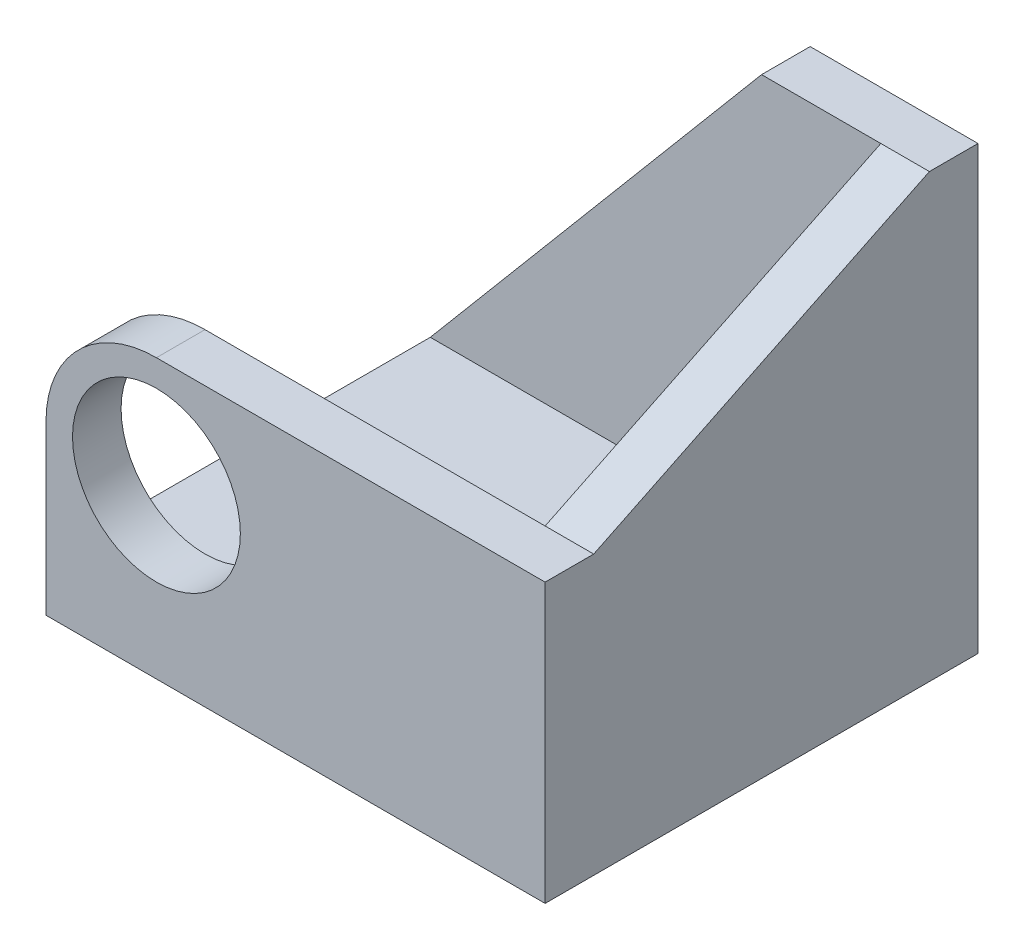
ISO-10303-21;
HEADER;
FILE_DESCRIPTION(('STEP AP214'),'2;1');
FILE_NAME('part.step','',(''),(''),'','','');
FILE_SCHEMA(('AUTOMOTIVE_DESIGN { 1 0 10303 214 1 1 1 1 }'));
ENDSEC;
DATA;
#1=APPLICATION_CONTEXT('core data for automotive mechanical design processes');
#2=APPLICATION_PROTOCOL_DEFINITION('international standard','automotive_design',2000,#1);
#3=PRODUCT_CONTEXT('',#1,'mechanical');
#4=PRODUCT('Part','Part','',(#3));
#5=PRODUCT_RELATED_PRODUCT_CATEGORY('part','',(#4));
#6=PRODUCT_DEFINITION_FORMATION('','',#4);
#7=PRODUCT_DEFINITION_CONTEXT('part definition',#1,'design');
#8=PRODUCT_DEFINITION('design','',#6,#7);
#9=PRODUCT_DEFINITION_SHAPE('','',#8);
#10=(LENGTH_UNIT() NAMED_UNIT(*) SI_UNIT(.MILLI.,.METRE.));
#11=(NAMED_UNIT(*) PLANE_ANGLE_UNIT() SI_UNIT($,.RADIAN.));
#12=(NAMED_UNIT(*) SI_UNIT($,.STERADIAN.) SOLID_ANGLE_UNIT());
#13=UNCERTAINTY_MEASURE_WITH_UNIT(LENGTH_MEASURE(1.E-05),#10,'distance_accuracy_value','');
#14=(GEOMETRIC_REPRESENTATION_CONTEXT(3) GLOBAL_UNCERTAINTY_ASSIGNED_CONTEXT((#13)) GLOBAL_UNIT_ASSIGNED_CONTEXT((#10,
#11,#12)) REPRESENTATION_CONTEXT('',''));
#15=CARTESIAN_POINT('',(0.,0.,0.));
#16=DIRECTION('',(0.,0.,1.));
#17=DIRECTION('',(1.,0.,0.));
#18=AXIS2_PLACEMENT_3D('',#15,#16,#17);
#19=CARTESIAN_POINT('',(25.,38.,0.));
#20=DIRECTION('',(0.,0.,1.));
#21=DIRECTION('',(1.,0.,0.));
#22=AXIS2_PLACEMENT_3D('',#19,#20,#21);
#23=PLANE('',#22);
#24=CARTESIAN_POINT('',(25.,38.,0.));
#25=DIRECTION('',(0.,0.,1.));
#26=DIRECTION('',(1.,0.,0.));
#27=AXIS2_PLACEMENT_3D('',#24,#25,#26);
#28=CIRCLE('',#27,19.);
#29=CARTESIAN_POINT('',(44.,38.,0.));
#30=VERTEX_POINT('',#29);
#31=EDGE_CURVE('E269',#30,#30,#28,.T.);
#32=ORIENTED_EDGE('',*,*,#31,.T.);
#33=EDGE_LOOP('',(#32));
#34=FACE_BOUND('',#33,.T.);
#35=DIRECTION('',(0.,-1.,0.));
#36=VECTOR('',#35,1.);
#37=CARTESIAN_POINT('',(67.,27.,0.));
#38=LINE('',#37,#36);
#39=CARTESIAN_POINT('',(67.,27.,0.));
#40=VERTEX_POINT('',#39);
#41=CARTESIAN_POINT('',(67.,11.,0.));
#42=VERTEX_POINT('',#41);
#43=EDGE_CURVE('E257',#40,#42,#38,.T.);
#44=ORIENTED_EDGE('',*,*,#43,.T.);
#45=DIRECTION('',(-1.,0.,0.));
#46=VECTOR('',#45,1.);
#47=CARTESIAN_POINT('',(0.,11.,0.));
#48=LINE('',#47,#46);
#49=CARTESIAN_POINT('',(0.,11.,0.));
#50=VERTEX_POINT('',#49);
#51=EDGE_CURVE('E164',#42,#50,#48,.T.);
#52=ORIENTED_EDGE('',*,*,#51,.T.);
#53=DIRECTION('',(0.,-1.,0.));
#54=VECTOR('',#53,1.);
#55=CARTESIAN_POINT('',(0.,0.,0.));
#56=LINE('',#55,#54);
#57=CARTESIAN_POINT('',(0.,38.,0.));
#58=VERTEX_POINT('',#57);
#59=EDGE_CURVE('E123',#58,#50,#56,.T.);
#60=ORIENTED_EDGE('',*,*,#59,.F.);
#61=CARTESIAN_POINT('',(25.,38.,0.));
#62=DIRECTION('',(0.,0.,1.));
#63=DIRECTION('',(1.,0.,0.));
#64=AXIS2_PLACEMENT_3D('',#61,#62,#63);
#65=CIRCLE('',#64,25.);
#66=CARTESIAN_POINT('',(25.,63.,0.));
#67=VERTEX_POINT('',#66);
#68=EDGE_CURVE('E81',#67,#58,#65,.T.);
#69=ORIENTED_EDGE('',*,*,#68,.F.);
#70=DIRECTION('',(-1.,0.,0.));
#71=VECTOR('',#70,1.);
#72=CARTESIAN_POINT('',(113.,63.,0.));
#73=LINE('',#72,#71);
#74=CARTESIAN_POINT('',(102.,63.,0.));
#75=VERTEX_POINT('',#74);
#76=EDGE_CURVE('E129',#75,#67,#73,.T.);
#77=ORIENTED_EDGE('',*,*,#76,.F.);
#78=DIRECTION('',(0.,-1.,0.));
#79=VECTOR('',#78,1.);
#80=CARTESIAN_POINT('',(102.,63.,0.));
#81=LINE('',#80,#79);
#82=CARTESIAN_POINT('',(102.,27.,0.));
#83=VERTEX_POINT('',#82);
#84=EDGE_CURVE('E185',#75,#83,#81,.T.);
#85=ORIENTED_EDGE('',*,*,#84,.T.);
#86=DIRECTION('',(1.,0.,0.));
#87=VECTOR('',#86,1.);
#88=CARTESIAN_POINT('',(102.,27.,0.));
#89=LINE('',#88,#87);
#90=EDGE_CURVE('E249',#40,#83,#89,.T.);
#91=ORIENTED_EDGE('',*,*,#90,.F.);
#92=EDGE_LOOP('',(#44,#52,#60,#69,#77,#85,#91));
#93=FACE_BOUND('',#92,.T.);
#94=ADVANCED_FACE('F44',(#34,#93),#23,.F.);
#95=CARTESIAN_POINT('',(102.,0.,0.));
#96=DIRECTION('',(1.,0.,0.));
#97=DIRECTION('',(0.,0.,-1.));
#98=AXIS2_PLACEMENT_3D('',#95,#96,#97);
#99=PLANE('',#98);
#100=DIRECTION('',(0.,0.,-1.));
#101=VECTOR('',#100,1.);
#102=CARTESIAN_POINT('',(102.,27.,-76.));
#103=LINE('',#102,#101);
#104=CARTESIAN_POINT('',(102.,27.,-76.));
#105=VERTEX_POINT('',#104);
#106=EDGE_CURVE('E256',#83,#105,#103,.T.);
#107=ORIENTED_EDGE('',*,*,#106,.F.);
#108=ORIENTED_EDGE('',*,*,#84,.F.);
#109=DIRECTION('',(0.,-0.437724250235496,0.899109270753991));
#110=VECTOR('',#109,1.);
#111=CARTESIAN_POINT('',(102.,100.,-76.));
#112=LINE('',#111,#110);
#113=CARTESIAN_POINT('',(102.,100.,-76.));
#114=VERTEX_POINT('',#113);
#115=EDGE_CURVE('E189',#114,#75,#112,.T.);
#116=ORIENTED_EDGE('',*,*,#115,.F.);
#117=DIRECTION('',(0.,1.,0.));
#118=VECTOR('',#117,1.);
#119=CARTESIAN_POINT('',(102.,0.,-76.));
#120=LINE('',#119,#118);
#121=EDGE_CURVE('E184',#105,#114,#120,.T.);
#122=ORIENTED_EDGE('',*,*,#121,.F.);
#123=EDGE_LOOP('',(#107,#108,#116,#122));
#124=FACE_BOUND('',#123,.T.);
#125=ADVANCED_FACE('F284',(#124),#99,.F.);
#126=CARTESIAN_POINT('',(0.,0.,-76.));
#127=DIRECTION('',(0.,0.,1.));
#128=DIRECTION('',(1.,0.,0.));
#129=AXIS2_PLACEMENT_3D('',#126,#127,#128);
#130=PLANE('',#129);
#131=DIRECTION('',(1.,0.,0.));
#132=VECTOR('',#131,1.);
#133=CARTESIAN_POINT('',(102.,11.,-76.));
#134=LINE('',#133,#132);
#135=CARTESIAN_POINT('',(0.,11.,-76.));
#136=VERTEX_POINT('',#135);
#137=CARTESIAN_POINT('',(67.,11.,-76.));
#138=VERTEX_POINT('',#137);
#139=EDGE_CURVE('E270',#136,#138,#134,.T.);
#140=ORIENTED_EDGE('',*,*,#139,.T.);
#141=DIRECTION('',(0.,-1.,0.));
#142=VECTOR('',#141,1.);
#143=CARTESIAN_POINT('',(67.,27.,-76.));
#144=LINE('',#143,#142);
#145=CARTESIAN_POINT('',(67.,27.,-76.));
#146=VERTEX_POINT('',#145);
#147=EDGE_CURVE('E58',#146,#138,#144,.T.);
#148=ORIENTED_EDGE('',*,*,#147,.F.);
#149=DIRECTION('',(-1.,0.,0.));
#150=VECTOR('',#149,1.);
#151=CARTESIAN_POINT('',(67.,27.,-76.));
#152=LINE('',#151,#150);
#153=EDGE_CURVE('E254',#105,#146,#152,.T.);
#154=ORIENTED_EDGE('',*,*,#153,.F.);
#155=ORIENTED_EDGE('',*,*,#121,.T.);
#156=DIRECTION('',(1.,0.,0.));
#157=VECTOR('',#156,1.);
#158=CARTESIAN_POINT('',(113.,100.,-76.));
#159=LINE('',#158,#157);
#160=CARTESIAN_POINT('',(75.,100.,-76.));
#161=VERTEX_POINT('',#160);
#162=EDGE_CURVE('E158',#161,#114,#159,.T.);
#163=ORIENTED_EDGE('',*,*,#162,.F.);
#164=DIRECTION('',(0.64440029083596,0.764688345125339,0.));
#165=VECTOR('',#164,1.);
#166=CARTESIAN_POINT('',(75.,100.,-76.));
#167=LINE('',#166,#165);
#168=EDGE_CURVE('E162',#136,#161,#167,.T.);
#169=ORIENTED_EDGE('',*,*,#168,.F.);
#170=EDGE_LOOP('',(#140,#148,#154,#155,#163,#169));
#171=FACE_BOUND('',#170,.T.);
#172=ADVANCED_FACE('F275',(#171),#130,.T.);
#173=CARTESIAN_POINT('',(0.,11.,0.));
#174=DIRECTION('',(0.,1.,0.));
#175=DIRECTION('',(0.,0.,1.));
#176=AXIS2_PLACEMENT_3D('',#173,#174,#175);
#177=PLANE('',#176);
#178=ORIENTED_EDGE('',*,*,#51,.F.);
#179=DIRECTION('',(0.,0.,1.));
#180=VECTOR('',#179,1.);
#181=CARTESIAN_POINT('',(67.,11.,0.));
#182=LINE('',#181,#180);
#183=EDGE_CURVE('E251',#138,#42,#182,.T.);
#184=ORIENTED_EDGE('',*,*,#183,.F.);
#185=ORIENTED_EDGE('',*,*,#139,.F.);
#186=DIRECTION('',(0.,0.,-1.));
#187=VECTOR('',#186,1.);
#188=CARTESIAN_POINT('',(0.,11.,-76.));
#189=LINE('',#188,#187);
#190=EDGE_CURVE('E227',#50,#136,#189,.T.);
#191=ORIENTED_EDGE('',*,*,#190,.F.);
#192=EDGE_LOOP('',(#178,#184,#185,#191));
#193=FACE_BOUND('',#192,.T.);
#194=ADVANCED_FACE('F273',(#193),#177,.T.);
#195=CARTESIAN_POINT('',(0.,0.,11.));
#196=DIRECTION('',(1.,0.,0.));
#197=DIRECTION('',(0.,1.,0.));
#198=AXIS2_PLACEMENT_3D('',#195,#196,#197);
#199=PLANE('',#198);
#200=ORIENTED_EDGE('',*,*,#59,.T.);
#201=ORIENTED_EDGE('',*,*,#190,.T.);
#202=DIRECTION('',(0.,0.,1.));
#203=VECTOR('',#202,1.);
#204=CARTESIAN_POINT('',(0.,11.,-87.));
#205=LINE('',#204,#203);
#206=CARTESIAN_POINT('',(0.,11.,-87.));
#207=VERTEX_POINT('',#206);
#208=EDGE_CURVE('E177',#207,#136,#205,.T.);
#209=ORIENTED_EDGE('',*,*,#208,.F.);
#210=DIRECTION('',(0.,1.,0.));
#211=VECTOR('',#210,1.);
#212=CARTESIAN_POINT('',(0.,0.,-87.));
#213=LINE('',#212,#211);
#214=CARTESIAN_POINT('',(0.,0.,-87.));
#215=VERTEX_POINT('',#214);
#216=EDGE_CURVE('E152',#215,#207,#213,.T.);
#217=ORIENTED_EDGE('',*,*,#216,.F.);
#218=DIRECTION('',(0.,0.,-1.));
#219=VECTOR('',#218,1.);
#220=CARTESIAN_POINT('',(0.,0.,11.));
#221=LINE('',#220,#219);
#222=CARTESIAN_POINT('',(0.,0.,11.));
#223=VERTEX_POINT('',#222);
#224=EDGE_CURVE('E11',#223,#215,#221,.T.);
#225=ORIENTED_EDGE('',*,*,#224,.F.);
#226=DIRECTION('',(0.,-1.,0.));
#227=VECTOR('',#226,1.);
#228=CARTESIAN_POINT('',(0.,0.,11.));
#229=LINE('',#228,#227);
#230=CARTESIAN_POINT('',(0.,38.,11.));
#231=VERTEX_POINT('',#230);
#232=EDGE_CURVE('E134',#231,#223,#229,.T.);
#233=ORIENTED_EDGE('',*,*,#232,.F.);
#234=DIRECTION('',(0.,0.,-1.));
#235=VECTOR('',#234,1.);
#236=CARTESIAN_POINT('',(0.,38.,11.));
#237=LINE('',#236,#235);
#238=EDGE_CURVE('E122',#231,#58,#237,.T.);
#239=ORIENTED_EDGE('',*,*,#238,.T.);
#240=EDGE_LOOP('',(#200,#201,#209,#217,#225,#233,#239));
#241=FACE_BOUND('',#240,.T.);
#242=ADVANCED_FACE('F50',(#241),#199,.F.);
#243=CARTESIAN_POINT('',(0.,0.,11.));
#244=DIRECTION('',(0.,1.,0.));
#245=DIRECTION('',(0.,0.,1.));
#246=AXIS2_PLACEMENT_3D('',#243,#244,#245);
#247=PLANE('',#246);
#248=ORIENTED_EDGE('',*,*,#224,.T.);
#249=DIRECTION('',(-1.,0.,0.));
#250=VECTOR('',#249,1.);
#251=CARTESIAN_POINT('',(113.,0.,-87.));
#252=LINE('',#251,#250);
#253=CARTESIAN_POINT('',(113.,0.,-87.));
#254=VERTEX_POINT('',#253);
#255=EDGE_CURVE('E143',#254,#215,#252,.T.);
#256=ORIENTED_EDGE('',*,*,#255,.F.);
#257=DIRECTION('',(0.,0.,-1.));
#258=VECTOR('',#257,1.);
#259=CARTESIAN_POINT('',(113.,0.,11.));
#260=LINE('',#259,#258);
#261=CARTESIAN_POINT('',(113.,0.,11.));
#262=VERTEX_POINT('',#261);
#263=EDGE_CURVE('E52',#262,#254,#260,.T.);
#264=ORIENTED_EDGE('',*,*,#263,.F.);
#265=DIRECTION('',(1.,0.,0.));
#266=VECTOR('',#265,1.);
#267=CARTESIAN_POINT('',(0.,0.,11.));
#268=LINE('',#267,#266);
#269=EDGE_CURVE('E91',#223,#262,#268,.T.);
#270=ORIENTED_EDGE('',*,*,#269,.F.);
#271=EDGE_LOOP('',(#248,#256,#264,#270));
#272=FACE_BOUND('',#271,.T.);
#273=ADVANCED_FACE('F147',(#272),#247,.F.);
#274=CARTESIAN_POINT('',(113.,0.,11.));
#275=DIRECTION('',(-1.,0.,0.));
#276=DIRECTION('',(0.,0.,1.));
#277=AXIS2_PLACEMENT_3D('',#274,#275,#276);
#278=PLANE('',#277);
#279=ORIENTED_EDGE('',*,*,#263,.T.);
#280=DIRECTION('',(0.,-1.,0.));
#281=VECTOR('',#280,1.);
#282=CARTESIAN_POINT('',(113.,0.,-87.));
#283=LINE('',#282,#281);
#284=CARTESIAN_POINT('',(113.,100.,-87.));
#285=VERTEX_POINT('',#284);
#286=EDGE_CURVE('E137',#285,#254,#283,.T.);
#287=ORIENTED_EDGE('',*,*,#286,.F.);
#288=DIRECTION('',(0.,0.,1.));
#289=VECTOR('',#288,1.);
#290=CARTESIAN_POINT('',(113.,100.,-87.));
#291=LINE('',#290,#289);
#292=CARTESIAN_POINT('',(113.,100.,-76.));
#293=VERTEX_POINT('',#292);
#294=EDGE_CURVE('E175',#285,#293,#291,.T.);
#295=ORIENTED_EDGE('',*,*,#294,.T.);
#296=DIRECTION('',(0.,-0.437724250235496,0.899109270753991));
#297=VECTOR('',#296,1.);
#298=CARTESIAN_POINT('',(113.,100.,-76.));
#299=LINE('',#298,#297);
#300=CARTESIAN_POINT('',(113.,63.,0.));
#301=VERTEX_POINT('',#300);
#302=EDGE_CURVE('E112',#293,#301,#299,.T.);
#303=ORIENTED_EDGE('',*,*,#302,.T.);
#304=DIRECTION('',(0.,0.,-1.));
#305=VECTOR('',#304,1.);
#306=CARTESIAN_POINT('',(113.,63.,11.));
#307=LINE('',#306,#305);
#308=CARTESIAN_POINT('',(113.,63.,11.));
#309=VERTEX_POINT('',#308);
#310=EDGE_CURVE('E109',#309,#301,#307,.T.);
#311=ORIENTED_EDGE('',*,*,#310,.F.);
#312=DIRECTION('',(0.,1.,0.));
#313=VECTOR('',#312,1.);
#314=CARTESIAN_POINT('',(113.,0.,11.));
#315=LINE('',#314,#313);
#316=EDGE_CURVE('E100',#262,#309,#315,.T.);
#317=ORIENTED_EDGE('',*,*,#316,.F.);
#318=EDGE_LOOP('',(#279,#287,#295,#303,#311,#317));
#319=FACE_BOUND('',#318,.T.);
#320=ADVANCED_FACE('F111',(#319),#278,.F.);
#321=CARTESIAN_POINT('',(113.,63.,11.));
#322=DIRECTION('',(0.,-1.,0.));
#323=DIRECTION('',(0.,0.,-1.));
#324=AXIS2_PLACEMENT_3D('',#321,#322,#323);
#325=PLANE('',#324);
#326=EDGE_CURVE('E128',#301,#75,#73,.T.);
#327=ORIENTED_EDGE('',*,*,#326,.T.);
#328=ORIENTED_EDGE('',*,*,#76,.T.);
#329=DIRECTION('',(0.,0.,-1.));
#330=VECTOR('',#329,1.);
#331=CARTESIAN_POINT('',(25.,63.,11.));
#332=LINE('',#331,#330);
#333=CARTESIAN_POINT('',(25.,63.,11.));
#334=VERTEX_POINT('',#333);
#335=EDGE_CURVE('E120',#334,#67,#332,.T.);
#336=ORIENTED_EDGE('',*,*,#335,.F.);
#337=DIRECTION('',(-1.,0.,0.));
#338=VECTOR('',#337,1.);
#339=CARTESIAN_POINT('',(113.,63.,11.));
#340=LINE('',#339,#338);
#341=EDGE_CURVE('E101',#309,#334,#340,.T.);
#342=ORIENTED_EDGE('',*,*,#341,.F.);
#343=ORIENTED_EDGE('',*,*,#310,.T.);
#344=EDGE_LOOP('',(#327,#328,#336,#342,#343));
#345=FACE_BOUND('',#344,.T.);
#346=ADVANCED_FACE('F118',(#345),#325,.F.);
#347=CARTESIAN_POINT('',(25.,38.,11.));
#348=DIRECTION('',(0.,0.,-1.));
#349=DIRECTION('',(-1.,0.,0.));
#350=AXIS2_PLACEMENT_3D('',#347,#348,#349);
#351=CYLINDRICAL_SURFACE('',#350,25.);
#352=ORIENTED_EDGE('',*,*,#68,.T.);
#353=ORIENTED_EDGE('',*,*,#238,.F.);
#354=CARTESIAN_POINT('',(25.,38.,11.));
#355=DIRECTION('',(0.,0.,1.));
#356=DIRECTION('',(1.,0.,0.));
#357=AXIS2_PLACEMENT_3D('',#354,#355,#356);
#358=CIRCLE('',#357,25.);
#359=EDGE_CURVE('E66',#334,#231,#358,.T.);
#360=ORIENTED_EDGE('',*,*,#359,.F.);
#361=ORIENTED_EDGE('',*,*,#335,.T.);
#362=EDGE_LOOP('',(#352,#353,#360,#361));
#363=FACE_BOUND('',#362,.T.);
#364=ADVANCED_FACE('F218',(#363),#351,.T.);
#365=CARTESIAN_POINT('',(25.,38.,11.));
#366=DIRECTION('',(0.,0.,1.));
#367=DIRECTION('',(1.,0.,0.));
#368=AXIS2_PLACEMENT_3D('',#365,#366,#367);
#369=PLANE('',#368);
#370=CARTESIAN_POINT('',(25.,38.,11.));
#371=DIRECTION('',(0.,0.,1.));
#372=DIRECTION('',(1.,0.,0.));
#373=AXIS2_PLACEMENT_3D('',#370,#371,#372);
#374=CIRCLE('',#373,19.);
#375=CARTESIAN_POINT('',(44.,38.,11.));
#376=VERTEX_POINT('',#375);
#377=EDGE_CURVE('E478',#376,#376,#374,.T.);
#378=ORIENTED_EDGE('',*,*,#377,.F.);
#379=EDGE_LOOP('',(#378));
#380=FACE_BOUND('',#379,.T.);
#381=ORIENTED_EDGE('',*,*,#232,.T.);
#382=ORIENTED_EDGE('',*,*,#269,.T.);
#383=ORIENTED_EDGE('',*,*,#316,.T.);
#384=ORIENTED_EDGE('',*,*,#341,.T.);
#385=ORIENTED_EDGE('',*,*,#359,.T.);
#386=EDGE_LOOP('',(#381,#382,#383,#384,#385));
#387=FACE_BOUND('',#386,.T.);
#388=ADVANCED_FACE('F103',(#380,#387),#369,.T.);
#389=CARTESIAN_POINT('',(102.,100.,-76.));
#390=DIRECTION('',(0.,0.899109270753991,0.437724250235496));
#391=DIRECTION('',(0.,-0.437724250235496,0.899109270753991));
#392=AXIS2_PLACEMENT_3D('',#389,#390,#391);
#393=PLANE('',#392);
#394=ORIENTED_EDGE('',*,*,#302,.F.);
#395=DIRECTION('',(1.,0.,0.));
#396=VECTOR('',#395,1.);
#397=CARTESIAN_POINT('',(102.,100.,-76.));
#398=LINE('',#397,#396);
#399=EDGE_CURVE('E126',#114,#293,#398,.T.);
#400=ORIENTED_EDGE('',*,*,#399,.F.);
#401=ORIENTED_EDGE('',*,*,#115,.T.);
#402=ORIENTED_EDGE('',*,*,#326,.F.);
#403=EDGE_LOOP('',(#394,#400,#401,#402));
#404=FACE_BOUND('',#403,.T.);
#405=ADVANCED_FACE('F217',(#404),#393,.T.);
#406=CARTESIAN_POINT('',(75.,100.,-87.));
#407=DIRECTION('',(0.764688345125339,-0.64440029083596,0.));
#408=DIRECTION('',(0.64440029083596,0.764688345125339,0.));
#409=AXIS2_PLACEMENT_3D('',#406,#407,#408);
#410=PLANE('',#409);
#411=ORIENTED_EDGE('',*,*,#168,.T.);
#412=DIRECTION('',(0.,0.,1.));
#413=VECTOR('',#412,1.);
#414=CARTESIAN_POINT('',(75.,100.,-87.));
#415=LINE('',#414,#413);
#416=CARTESIAN_POINT('',(75.,100.,-87.));
#417=VERTEX_POINT('',#416);
#418=EDGE_CURVE('E176',#417,#161,#415,.T.);
#419=ORIENTED_EDGE('',*,*,#418,.F.);
#420=DIRECTION('',(0.64440029083596,0.764688345125339,0.));
#421=VECTOR('',#420,1.);
#422=CARTESIAN_POINT('',(75.,100.,-87.));
#423=LINE('',#422,#421);
#424=EDGE_CURVE('E169',#207,#417,#423,.T.);
#425=ORIENTED_EDGE('',*,*,#424,.F.);
#426=ORIENTED_EDGE('',*,*,#208,.T.);
#427=EDGE_LOOP('',(#411,#419,#425,#426));
#428=FACE_BOUND('',#427,.T.);
#429=ADVANCED_FACE('F316',(#428),#410,.F.);
#430=CARTESIAN_POINT('',(113.,100.,-87.));
#431=DIRECTION('',(0.,-1.,0.));
#432=DIRECTION('',(0.,0.,-1.));
#433=AXIS2_PLACEMENT_3D('',#430,#431,#432);
#434=PLANE('',#433);
#435=ORIENTED_EDGE('',*,*,#162,.T.);
#436=ORIENTED_EDGE('',*,*,#399,.T.);
#437=ORIENTED_EDGE('',*,*,#294,.F.);
#438=DIRECTION('',(1.,0.,0.));
#439=VECTOR('',#438,1.);
#440=CARTESIAN_POINT('',(113.,100.,-87.));
#441=LINE('',#440,#439);
#442=EDGE_CURVE('E156',#417,#285,#441,.T.);
#443=ORIENTED_EDGE('',*,*,#442,.F.);
#444=ORIENTED_EDGE('',*,*,#418,.T.);
#445=EDGE_LOOP('',(#435,#436,#437,#443,#444));
#446=FACE_BOUND('',#445,.T.);
#447=ADVANCED_FACE('F321',(#446),#434,.F.);
#448=CARTESIAN_POINT('',(0.,0.,-87.));
#449=DIRECTION('',(0.,0.,1.));
#450=DIRECTION('',(1.,0.,0.));
#451=AXIS2_PLACEMENT_3D('',#448,#449,#450);
#452=PLANE('',#451);
#453=ORIENTED_EDGE('',*,*,#286,.T.);
#454=ORIENTED_EDGE('',*,*,#255,.T.);
#455=ORIENTED_EDGE('',*,*,#216,.T.);
#456=ORIENTED_EDGE('',*,*,#424,.T.);
#457=ORIENTED_EDGE('',*,*,#442,.T.);
#458=EDGE_LOOP('',(#453,#454,#455,#456,#457));
#459=FACE_BOUND('',#458,.T.);
#460=ADVANCED_FACE('F151',(#459),#452,.F.);
#461=CARTESIAN_POINT('',(67.,27.,0.));
#462=DIRECTION('',(1.,0.,0.));
#463=DIRECTION('',(0.,0.,-1.));
#464=AXIS2_PLACEMENT_3D('',#461,#462,#463);
#465=PLANE('',#464);
#466=ORIENTED_EDGE('',*,*,#183,.T.);
#467=ORIENTED_EDGE('',*,*,#43,.F.);
#468=DIRECTION('',(0.,0.,1.));
#469=VECTOR('',#468,1.);
#470=CARTESIAN_POINT('',(67.,27.,0.));
#471=LINE('',#470,#469);
#472=EDGE_CURVE('E246',#146,#40,#471,.T.);
#473=ORIENTED_EDGE('',*,*,#472,.F.);
#474=ORIENTED_EDGE('',*,*,#147,.T.);
#475=EDGE_LOOP('',(#466,#467,#473,#474));
#476=FACE_BOUND('',#475,.T.);
#477=ADVANCED_FACE('F260',(#476),#465,.F.);
#478=CARTESIAN_POINT('',(0.,27.,0.));
#479=DIRECTION('',(0.,-1.,0.));
#480=DIRECTION('',(0.,0.,-1.));
#481=AXIS2_PLACEMENT_3D('',#478,#479,#480);
#482=PLANE('',#481);
#483=ORIENTED_EDGE('',*,*,#472,.T.);
#484=ORIENTED_EDGE('',*,*,#90,.T.);
#485=ORIENTED_EDGE('',*,*,#106,.T.);
#486=ORIENTED_EDGE('',*,*,#153,.T.);
#487=EDGE_LOOP('',(#483,#484,#485,#486));
#488=FACE_BOUND('',#487,.T.);
#489=ADVANCED_FACE('F247',(#488),#482,.F.);
#490=CARTESIAN_POINT('',(25.,38.,0.));
#491=DIRECTION('',(0.,0.,1.));
#492=DIRECTION('',(1.,0.,0.));
#493=AXIS2_PLACEMENT_3D('',#490,#491,#492);
#494=CYLINDRICAL_SURFACE('',#493,19.);
#495=ORIENTED_EDGE('',*,*,#31,.F.);
#496=EDGE_LOOP('',(#495));
#497=FACE_BOUND('',#496,.T.);
#498=ORIENTED_EDGE('',*,*,#377,.T.);
#499=EDGE_LOOP('',(#498));
#500=FACE_BOUND('',#499,.T.);
#501=ADVANCED_FACE('F443',(#497,#500),#494,.F.);
#502=CLOSED_SHELL('',(#94,#125,#172,#194,#242,#273,#320,#346,#364,#388,#405,#429,#447,#460,#477,
#489,#501));
#503=MANIFOLD_SOLID_BREP('B2',#502);
#504=ADVANCED_BREP_SHAPE_REPRESENTATION('',(#18,#503),#14);
#505=SHAPE_DEFINITION_REPRESENTATION(#9,#504);
ENDSEC;
END-ISO-10303-21;
